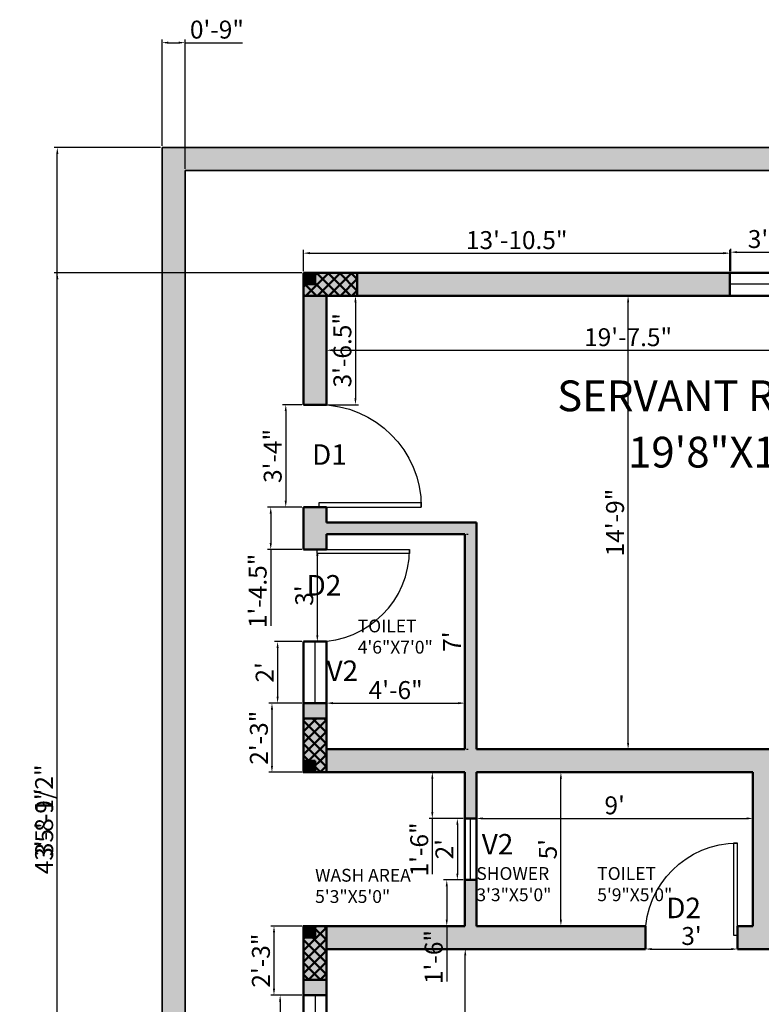
# Model space of a CAD drawing. Units: inches. Extents: x 1749 to 3550, y 1117 to 2383.
# Tile 7 of 15: x 1749 to 2038, y 1993 to 2377. Entities that reach past the tile are written whole.
import ezdxf

# ---------------------------------------------------------------- set-up
doc = ezdxf.new("R2010")
doc.units = ezdxf.units.IN
for name, color, linetype, lineweight in [('A-ANNO-DIMS', 2, 'Continuous', 18), ('A-ANNO-TEXT', 3, 'Continuous', 18), ('A-AREA-IDEN', 7, 'Continuous', 18), ('A-COLS', 10, 'Continuous', 50), ('A-DOOR', 30, 'Continuous', 25), ('A-GLAZ', 4, 'Continuous', 25), ('A-WALL', 7, 'Continuous', 50), ('A-WALL-PATT', 8, 'Continuous', 13), ('C-PROP', 8, 'Continuous', 35)]:
    doc.layers.add(name, color=color, linetype=linetype, lineweight=lineweight)
doc.styles.get("Standard").update_dxf_attribs({"font": 'arial.ttf'})
doc.dimstyles.new('ISO-25', dxfattribs={"dimtxt": 7, "dimasz": 2.5, "dimexe": 1.25, "dimexo": 0.625, "dimtad": 1, "dimdec": 1, "dimlunit": 3, "dimtxsty": 'Standard', "dimcen": 2.5, "dimadec": 0, "dimazin": 0, "dimtfac": 1, "dimtdec": 1, "dimtmove": 0, "dimatfit": 3, "dimfxl": 1, "dimarcsym": 0})

# ---------------------------------------------------------------- blocks, each defined once
blk = doc.blocks.new('*U2')
for p, q in [((0, 0), (0, -6)), ((40, 0), (40, -6))]:
    blk.add_line(p, q)
blk.add_lwpolyline([(0, 0), (0, 40), (1.75, 40), (1.75, 0)], close=True)
blk.add_arc((0, 0), 40, 0, 90)
blk = doc.blocks.new('*U3')
for p, q in [((0, 0), (0, -6)), ((40, 0), (40, -6))]:
    blk.add_line(p, q)
blk.add_lwpolyline([(0, 0), (0, 40), (1.75, 40), (1.75, 0)], close=True)
blk.add_arc((0, 0), 40, 0, 90)
blk = doc.blocks.new('*D4')
at = {"layer": 'A-ANNO-DIMS', "color": 0, "lineweight": -2, "transparency": 16777216}
for p, q in [((1994.36, 2269.66), (1985.1, 2269.66)), ((1986.35, 2095.16), (1986.35, 2267.16)), ((1994.36, 2092.66), (1985.1, 2092.66))]:
    blk.add_line(p, q, dxfattribs=at)
at = {"layer": 'A-ANNO-DIMS', "color": 0, "transparency": 16777216}
for points in [[(1985.94, 2267.16), (1986.77, 2267.16), (1986.35, 2269.66)], [(1985.94, 2095.16), (1986.77, 2095.16), (1986.35, 2092.66)]]:
    blk.add_solid(points, dxfattribs=at)
at = {"layer": 'Defpoints', "color": 0, "transparency": 16777216}
for p in [(1986.35, 2269.66), (1994.99, 2269.66), (1994.99, 2092.66)]:
    blk.add_point(p, dxfattribs=at)
at = {"layer": 'A-ANNO-DIMS', "color": 0, "transparency": 16777216, "insert": (1982.16, 2181.16), "char_height": 7, "attachment_point": 5, "rotation": 90}
blk.add_mtext('14\'-9"', dxfattribs=at)
blk = doc.blocks.new('*D5')
at = {"layer": 'A-ANNO-DIMS', "color": 0, "lineweight": -2, "transparency": 16777216}
for p, q in [((1868.6, 2249.04), (1868.6, 2249.66)), ((2104.1, 2249.04), (2104.1, 2249.66)), ((1871.1, 2248.41), (2101.6, 2248.41))]:
    blk.add_line(p, q, dxfattribs=at)
at = {"layer": 'A-ANNO-DIMS', "color": 0, "transparency": 16777216}
for points in [[(1871.1, 2248.83), (1871.1, 2247.99), (1868.6, 2248.41)], [(2101.6, 2248.83), (2101.6, 2247.99), (2104.1, 2248.41)]]:
    blk.add_solid(points, dxfattribs=at)
at = {"layer": 'Defpoints', "color": 0, "transparency": 16777216}
for p in [(1868.6, 2248.41), (2104.1, 2248.41), (2104.1, 2248.41)]:
    blk.add_point(p, dxfattribs=at)
at = {"layer": 'A-ANNO-DIMS', "color": 0, "transparency": 16777216, "insert": (1986.35, 2252.61), "char_height": 7, "attachment_point": 5}
blk.add_mtext('19\'-7.5"', dxfattribs=at)
blk = doc.blocks.new('*D6')
at = {"layer": 'A-ANNO-DIMS', "color": 0, "lineweight": -2, "transparency": 16777216}
for p, q in [((1923.39, 2014.66), (1924.02, 2014.66)), ((1922.77, 1861.16), (1922.77, 2012.16)), ((1923.39, 1858.66), (1924.02, 1858.66))]:
    blk.add_line(p, q, dxfattribs=at)
at = {"layer": 'A-ANNO-DIMS', "color": 0, "transparency": 16777216}
for points in [[(1922.35, 2012.16), (1923.18, 2012.16), (1922.77, 2014.66)], [(1922.35, 1861.16), (1923.18, 1861.16), (1922.77, 1858.66)]]:
    blk.add_solid(points, dxfattribs=at)
at = {"layer": 'Defpoints', "color": 0, "transparency": 16777216}
for p in [(1922.77, 2014.66), (1922.77, 2014.66), (1922.77, 1858.66)]:
    blk.add_point(p, dxfattribs=at)
at = {"layer": 'A-ANNO-DIMS', "color": 0, "transparency": 16777216, "insert": (1918.57, 1936.66), "char_height": 7, "attachment_point": 5, "rotation": 90}
blk.add_mtext("13'", dxfattribs=at)
blk = doc.blocks.new('*D8')
at = {"layer": 'A-ANNO-DIMS', "color": 0, "lineweight": -2, "transparency": 16777216}
for p, q in [((1960.73, 2083.66), (1961.35, 2083.66)), ((1960.1, 2026.16), (1960.1, 2081.16)), ((1960.73, 2023.66), (1961.35, 2023.66))]:
    blk.add_line(p, q, dxfattribs=at)
at = {"layer": 'A-ANNO-DIMS', "color": 0, "transparency": 16777216}
for points in [[(1959.69, 2081.16), (1960.52, 2081.16), (1960.1, 2083.66)], [(1959.69, 2026.16), (1960.52, 2026.16), (1960.1, 2023.66)]]:
    blk.add_solid(points, dxfattribs=at)
at = {"layer": 'Defpoints', "color": 0, "transparency": 16777216}
for p in [(1960.1, 2083.66), (1960.1, 2083.66), (1960.1, 2023.66)]:
    blk.add_point(p, dxfattribs=at)
at = {"layer": 'A-ANNO-DIMS', "color": 0, "transparency": 16777216, "insert": (1955.92, 2053.66), "char_height": 7, "attachment_point": 5, "rotation": 90}
blk.add_mtext("5'", dxfattribs=at)
blk = doc.blocks.new('*D9')
at = {"layer": 'A-ANNO-DIMS', "color": 0, "lineweight": -2, "transparency": 16777216}
for p, q in [((1927.1, 2066.29), (1927.1, 2066.91)), ((1929.6, 2065.66), (2032.6, 2065.66)), ((2035.1, 2066.29), (2035.1, 2066.91))]:
    blk.add_line(p, q, dxfattribs=at)
at = {"layer": 'A-ANNO-DIMS', "color": 0, "transparency": 16777216}
for points in [[(1929.6, 2066.08), (1929.6, 2065.24), (1927.1, 2065.66)], [(2032.6, 2066.08), (2032.6, 2065.24), (2035.1, 2065.66)]]:
    blk.add_solid(points, dxfattribs=at)
at = {"layer": 'Defpoints', "color": 0, "transparency": 16777216}
for p in [(1927.1, 2065.66), (2035.1, 2065.66), (2035.1, 2065.66)]:
    blk.add_point(p, dxfattribs=at)
at = {"layer": 'A-ANNO-DIMS', "color": 0, "transparency": 16777216, "insert": (1981.1, 2069.86), "char_height": 7, "attachment_point": 5}
blk.add_mtext("9'", dxfattribs=at)
blk = doc.blocks.new('*D10')
at = {"layer": 'A-ANNO-DIMS', "color": 0, "lineweight": -2, "transparency": 16777216}
for p, q in [((1923.23, 2176.66), (1923.85, 2176.66)), ((1922.6, 2095.16), (1922.6, 2174.16)), ((1923.23, 2092.66), (1923.85, 2092.66))]:
    blk.add_line(p, q, dxfattribs=at)
at = {"layer": 'A-ANNO-DIMS', "color": 0, "transparency": 16777216}
for points in [[(1922.19, 2174.16), (1923.02, 2174.16), (1922.6, 2176.66)], [(1922.19, 2095.16), (1923.02, 2095.16), (1922.6, 2092.66)]]:
    blk.add_solid(points, dxfattribs=at)
at = {"layer": 'Defpoints', "color": 0, "transparency": 16777216}
for p in [(1922.6, 2176.66), (1922.6, 2176.66), (1922.6, 2092.66)]:
    blk.add_point(p, dxfattribs=at)
at = {"layer": 'A-ANNO-DIMS', "color": 0, "transparency": 16777216, "insert": (1918.48, 2134.66), "char_height": 7, "attachment_point": 5, "rotation": 90}
blk.add_mtext("7'", dxfattribs=at)
blk = doc.blocks.new('*D11')
at = {"layer": 'A-ANNO-DIMS', "color": 0, "lineweight": -2, "transparency": 16777216}
for p, q in [((1868.6, 2111.29), (1868.6, 2111.91)), ((1871.1, 2110.66), (1920.1, 2110.66)), ((1922.6, 2111.29), (1922.6, 2111.91))]:
    blk.add_line(p, q, dxfattribs=at)
at = {"layer": 'A-ANNO-DIMS', "color": 0, "transparency": 16777216}
for points in [[(1871.1, 2111.08), (1871.1, 2110.24), (1868.6, 2110.66)], [(1920.1, 2111.08), (1920.1, 2110.24), (1922.6, 2110.66)]]:
    blk.add_solid(points, dxfattribs=at)
at = {"layer": 'Defpoints', "color": 0, "transparency": 16777216}
for p in [(1868.6, 2110.66), (1922.6, 2110.66), (1922.6, 2110.66)]:
    blk.add_point(p, dxfattribs=at)
at = {"layer": 'A-ANNO-DIMS', "color": 0, "transparency": 16777216, "insert": (1895.6, 2114.86), "char_height": 7, "attachment_point": 5}
blk.add_mtext('4\'-6"', dxfattribs=at)
blk = doc.blocks.new('*D75')
at = {"layer": 'A-ANNO-DIMS', "color": 0, "lineweight": -2, "ltscale": 0.5, "transparency": 16777216}
for p, q in [((1859.6, 2279.29), (1859.6, 2287.56)), ((2026.1, 2279.29), (2026.1, 2287.56)), ((1862.1, 2286.31), (2023.6, 2286.31))]:
    blk.add_line(p, q, dxfattribs=at)
at = {"layer": 'A-ANNO-DIMS', "color": 0, "ltscale": 0.5, "transparency": 16777216}
for points in [[(1862.1, 2286.73), (1862.1, 2285.9), (1859.6, 2286.31)], [(2023.6, 2286.73), (2023.6, 2285.9), (2026.1, 2286.31)]]:
    blk.add_solid(points, dxfattribs=at)
at = {"layer": 'Defpoints', "color": 0, "ltscale": 0.5, "transparency": 16777216}
for p in [(2026.1, 2286.31), (1859.6, 2278.66), (2026.1, 2278.66)]:
    blk.add_point(p, dxfattribs=at)
at = {"layer": 'A-ANNO-DIMS', "color": 0, "ltscale": 0.5, "transparency": 16777216, "insert": (1942.85, 2290.51), "char_height": 7, "attachment_point": 5}
blk.add_mtext('13\'-10.5"', dxfattribs=at)
blk = doc.blocks.new('*D76')
at = {"layer": 'A-ANNO-DIMS', "color": 0, "lineweight": -2, "ltscale": 0.5, "transparency": 16777216}
for p, q in [((2026.42, 2279.29), (2026.42, 2287.96)), ((2074.1, 2279.29), (2074.1, 2287.96)), ((2028.92, 2286.71), (2071.6, 2286.71))]:
    blk.add_line(p, q, dxfattribs=at)
at = {"layer": 'A-ANNO-DIMS', "color": 0, "ltscale": 0.5, "transparency": 16777216}
for points in [[(2028.92, 2287.12), (2028.92, 2286.29), (2026.42, 2286.71)], [(2071.6, 2287.12), (2071.6, 2286.29), (2074.1, 2286.71)]]:
    blk.add_solid(points, dxfattribs=at)
at = {"layer": 'Defpoints', "color": 0, "ltscale": 0.5, "transparency": 16777216}
for p in [(2074.1, 2286.71), (2026.42, 2278.66), (2074.1, 2278.66)]:
    blk.add_point(p, dxfattribs=at)
at = {"layer": 'A-ANNO-DIMS', "color": 0, "ltscale": 0.5, "transparency": 16777216, "insert": (2050.26, 2290.91), "char_height": 7, "attachment_point": 5}
blk.add_mtext('3\'-11.7"', dxfattribs=at)
blk = doc.blocks.new('*D78')
at = {"layer": 'A-ANNO-DIMS', "color": 0, "lineweight": -2, "ltscale": 0.5, "transparency": 16777216}
for p, q in [((1869.23, 2269.66), (1881.14, 2269.66)), ((1879.89, 2267.16), (1879.89, 2229.66)), ((1869.23, 2227.16), (1881.14, 2227.16))]:
    blk.add_line(p, q, dxfattribs=at)
at = {"layer": 'A-ANNO-DIMS', "color": 0, "ltscale": 0.5, "transparency": 16777216}
for points in [[(1879.48, 2267.16), (1880.31, 2267.16), (1879.89, 2269.66)], [(1879.48, 2229.66), (1880.31, 2229.66), (1879.89, 2227.16)]]:
    blk.add_solid(points, dxfattribs=at)
at = {"layer": 'Defpoints', "color": 0, "ltscale": 0.5, "transparency": 16777216}
for p in [(1868.6, 2269.66), (1868.6, 2227.16), (1879.89, 2227.16)]:
    blk.add_point(p, dxfattribs=at)
at = {"layer": 'A-ANNO-DIMS', "color": 0, "ltscale": 0.5, "transparency": 16777216, "insert": (1875.69, 2248.41), "char_height": 7, "attachment_point": 5, "rotation": 90}
blk.add_mtext('3\'-6.5"', dxfattribs=at)
blk = doc.blocks.new('*D79')
at = {"layer": 'A-ANNO-DIMS', "color": 0, "lineweight": -2, "ltscale": 0.5, "transparency": 16777216}
for p, q in [((1858.98, 2227.16), (1851.43, 2227.16)), ((1852.68, 2224.66), (1852.68, 2189.66)), ((1858.98, 2187.16), (1851.43, 2187.16))]:
    blk.add_line(p, q, dxfattribs=at)
at = {"layer": 'A-ANNO-DIMS', "color": 0, "ltscale": 0.5, "transparency": 16777216}
for points in [[(1852.26, 2224.66), (1853.09, 2224.66), (1852.68, 2227.16)], [(1852.26, 2189.66), (1853.09, 2189.66), (1852.68, 2187.16)]]:
    blk.add_solid(points, dxfattribs=at)
at = {"layer": 'Defpoints', "color": 0, "ltscale": 0.5, "transparency": 16777216}
for p in [(1859.61, 2227.16), (1852.68, 2187.16), (1859.6, 2187.16)]:
    blk.add_point(p, dxfattribs=at)
at = {"layer": 'A-ANNO-DIMS', "color": 0, "ltscale": 0.5, "transparency": 16777216, "insert": (1848.48, 2207.16), "char_height": 7, "attachment_point": 5, "rotation": 90}
blk.add_mtext('3\'-4"', dxfattribs=at)
blk = doc.blocks.new('*D80')
at = {"layer": 'A-ANNO-DIMS', "color": 0, "lineweight": -2, "ltscale": 0.5, "transparency": 16777216}
for p, q in [((1858.98, 2187.16), (1845.56, 2187.16)), ((1846.81, 2184.66), (1846.81, 2173.16)), ((1858.98, 2170.66), (1845.56, 2170.66)), ((1846.81, 2170.66), (1846.81, 2140.81))]:
    blk.add_line(p, q, dxfattribs=at)
at = {"layer": 'A-ANNO-DIMS', "color": 0, "ltscale": 0.5, "transparency": 16777216}
for points in [[(1846.39, 2184.66), (1847.23, 2184.66), (1846.81, 2187.16)], [(1846.39, 2173.16), (1847.23, 2173.16), (1846.81, 2170.66)]]:
    blk.add_solid(points, dxfattribs=at)
at = {"layer": 'Defpoints', "color": 0, "ltscale": 0.5, "transparency": 16777216}
for p in [(1859.6, 2187.16), (1846.81, 2170.66), (1859.6, 2170.66)]:
    blk.add_point(p, dxfattribs=at)
at = {"layer": 'A-ANNO-DIMS', "color": 0, "ltscale": 0.5, "transparency": 16777216, "insert": (1842.61, 2154.48), "char_height": 7, "attachment_point": 5, "rotation": 90}
blk.add_mtext('1\'-4.5"', dxfattribs=at)
blk = doc.blocks.new('*D81')
at = {"layer": 'A-ANNO-DIMS', "color": 0, "lineweight": -2, "ltscale": 0.5, "transparency": 16777216}
for p, q in [((1860.23, 2170.66), (1866.25, 2170.66)), ((1865, 2168.16), (1865, 2137.16)), ((1860.23, 2134.66), (1866.25, 2134.66))]:
    blk.add_line(p, q, dxfattribs=at)
at = {"layer": 'A-ANNO-DIMS', "color": 0, "ltscale": 0.5, "transparency": 16777216}
for points in [[(1864.59, 2168.16), (1865.42, 2168.16), (1865, 2170.66)], [(1864.59, 2137.16), (1865.42, 2137.16), (1865, 2134.66)]]:
    blk.add_solid(points, dxfattribs=at)
at = {"layer": 'Defpoints', "color": 0, "ltscale": 0.5, "transparency": 16777216}
for p in [(1859.6, 2170.66), (1859.6, 2134.66), (1865, 2134.66)]:
    blk.add_point(p, dxfattribs=at)
at = {"layer": 'A-ANNO-DIMS', "color": 0, "ltscale": 0.5, "transparency": 16777216, "insert": (1860.8, 2152.66), "char_height": 7, "attachment_point": 5, "rotation": 90}
blk.add_mtext("3'", dxfattribs=at)
blk = doc.blocks.new('*D82')
at = {"layer": 'A-ANNO-DIMS', "color": 0, "lineweight": -2, "ltscale": 0.5, "transparency": 16777216}
for p, q in [((1858.98, 2134.66), (1848.24, 2134.66)), ((1849.49, 2132.16), (1849.49, 2113.16)), ((1858.98, 2110.66), (1848.24, 2110.66))]:
    blk.add_line(p, q, dxfattribs=at)
at = {"layer": 'A-ANNO-DIMS', "color": 0, "ltscale": 0.5, "transparency": 16777216}
for points in [[(1849.08, 2132.16), (1849.91, 2132.16), (1849.49, 2134.66)], [(1849.08, 2113.16), (1849.91, 2113.16), (1849.49, 2110.66)]]:
    blk.add_solid(points, dxfattribs=at)
at = {"layer": 'Defpoints', "color": 0, "ltscale": 0.5, "transparency": 16777216}
for p in [(1859.6, 2134.66), (1849.49, 2110.66), (1859.6, 2110.66)]:
    blk.add_point(p, dxfattribs=at)
at = {"layer": 'A-ANNO-DIMS', "color": 0, "ltscale": 0.5, "transparency": 16777216, "insert": (1845.35, 2122.66), "char_height": 7, "attachment_point": 5, "rotation": 90}
blk.add_mtext("2'", dxfattribs=at)
blk = doc.blocks.new('*D83')
at = {"layer": 'A-ANNO-DIMS', "color": 0, "lineweight": -2, "ltscale": 0.5, "transparency": 16777216}
for p, q in [((1858.98, 2110.66), (1846.04, 2110.66)), ((1847.29, 2108.16), (1847.29, 2086.16)), ((1858.98, 2083.66), (1846.04, 2083.66))]:
    blk.add_line(p, q, dxfattribs=at)
at = {"layer": 'A-ANNO-DIMS', "color": 0, "ltscale": 0.5, "transparency": 16777216}
for points in [[(1846.87, 2108.16), (1847.71, 2108.16), (1847.29, 2110.66)], [(1846.87, 2086.16), (1847.71, 2086.16), (1847.29, 2083.66)]]:
    blk.add_solid(points, dxfattribs=at)
at = {"layer": 'Defpoints', "color": 0, "ltscale": 0.5, "transparency": 16777216}
for p in [(1859.6, 2110.66), (1847.29, 2083.66), (1859.6, 2083.66)]:
    blk.add_point(p, dxfattribs=at)
at = {"layer": 'A-ANNO-DIMS', "color": 0, "ltscale": 0.5, "transparency": 16777216, "insert": (1843.09, 2097.16), "char_height": 7, "attachment_point": 5, "rotation": 90}
blk.add_mtext('2\'-3"', dxfattribs=at)
blk = doc.blocks.new('*D84')
at = {"layer": 'A-ANNO-DIMS', "color": 0, "lineweight": -2, "ltscale": 0.5, "transparency": 16777216}
for p, q in [((1921.98, 2083.66), (1908.65, 2083.66)), ((1909.9, 2081.16), (1909.9, 2068.16)), ((1921.98, 2065.66), (1908.65, 2065.66)), ((1909.9, 2065.66), (1909.9, 2043.96))]:
    blk.add_line(p, q, dxfattribs=at)
at = {"layer": 'A-ANNO-DIMS', "color": 0, "ltscale": 0.5, "transparency": 16777216}
for points in [[(1909.49, 2081.16), (1910.32, 2081.16), (1909.9, 2083.66)], [(1909.49, 2068.16), (1910.32, 2068.16), (1909.9, 2065.66)]]:
    blk.add_solid(points, dxfattribs=at)
at = {"layer": 'Defpoints', "color": 0, "ltscale": 0.5, "transparency": 16777216}
for p in [(1922.6, 2083.66), (1909.9, 2065.66), (1922.6, 2065.66)]:
    blk.add_point(p, dxfattribs=at)
at = {"layer": 'A-ANNO-DIMS', "color": 0, "ltscale": 0.5, "transparency": 16777216, "insert": (1905.7, 2053.56), "char_height": 7, "attachment_point": 5, "rotation": 90}
blk.add_mtext('1\'-6"', dxfattribs=at)
blk = doc.blocks.new('*D85')
at = {"layer": 'A-ANNO-DIMS', "color": 0, "lineweight": -2, "ltscale": 0.5, "transparency": 16777216}
for p, q in [((1921.98, 2065.66), (1918.43, 2065.66)), ((1919.68, 2063.16), (1919.68, 2044.16)), ((1921.98, 2041.66), (1918.43, 2041.66))]:
    blk.add_line(p, q, dxfattribs=at)
at = {"layer": 'A-ANNO-DIMS', "color": 0, "ltscale": 0.5, "transparency": 16777216}
for points in [[(1919.26, 2063.16), (1920.1, 2063.16), (1919.68, 2065.66)], [(1919.26, 2044.16), (1920.1, 2044.16), (1919.68, 2041.66)]]:
    blk.add_solid(points, dxfattribs=at)
at = {"layer": 'Defpoints', "color": 0, "ltscale": 0.5, "transparency": 16777216}
for p in [(1922.6, 2065.66), (1919.68, 2041.66), (1922.6, 2041.66)]:
    blk.add_point(p, dxfattribs=at)
at = {"layer": 'A-ANNO-DIMS', "color": 0, "ltscale": 0.5, "transparency": 16777216, "insert": (1915.54, 2053.66), "char_height": 7, "attachment_point": 5, "rotation": 90}
blk.add_mtext("2'", dxfattribs=at)
blk = doc.blocks.new('*D86')
at = {"layer": 'A-ANNO-DIMS', "color": 0, "lineweight": -2, "ltscale": 0.5, "transparency": 16777216}
for p, q in [((1921.98, 2041.66), (1914.3, 2041.66)), ((1915.55, 2039.16), (1915.55, 2026.16)), ((1921.98, 2023.66), (1914.3, 2023.66)), ((1915.55, 2023.66), (1915.55, 2001.96))]:
    blk.add_line(p, q, dxfattribs=at)
at = {"layer": 'A-ANNO-DIMS', "color": 0, "ltscale": 0.5, "transparency": 16777216}
for points in [[(1915.14, 2039.16), (1915.97, 2039.16), (1915.55, 2041.66)], [(1915.14, 2026.16), (1915.97, 2026.16), (1915.55, 2023.66)]]:
    blk.add_solid(points, dxfattribs=at)
at = {"layer": 'Defpoints', "color": 0, "ltscale": 0.5, "transparency": 16777216}
for p in [(1922.6, 2041.66), (1915.55, 2023.66), (1922.6, 2023.66)]:
    blk.add_point(p, dxfattribs=at)
at = {"layer": 'A-ANNO-DIMS', "color": 0, "ltscale": 0.5, "transparency": 16777216, "insert": (1911.35, 2011.56), "char_height": 7, "attachment_point": 5, "rotation": 90}
blk.add_mtext('1\'-6"', dxfattribs=at)
blk = doc.blocks.new('*D87')
at = {"layer": 'A-ANNO-DIMS', "color": 0, "lineweight": -2, "ltscale": 0.5, "transparency": 16777216}
for p, q in [((1858.98, 2023.66), (1846.83, 2023.66)), ((1848.08, 2021.16), (1848.08, 1999.16)), ((1858.98, 1996.66), (1846.83, 1996.66))]:
    blk.add_line(p, q, dxfattribs=at)
at = {"layer": 'A-ANNO-DIMS', "color": 0, "ltscale": 0.5, "transparency": 16777216}
for points in [[(1847.66, 2021.16), (1848.5, 2021.16), (1848.08, 2023.66)], [(1847.66, 1999.16), (1848.5, 1999.16), (1848.08, 1996.66)]]:
    blk.add_solid(points, dxfattribs=at)
at = {"layer": 'Defpoints', "color": 0, "ltscale": 0.5, "transparency": 16777216}
for p in [(1859.6, 2023.66), (1848.08, 1996.66), (1859.6, 1996.66)]:
    blk.add_point(p, dxfattribs=at)
at = {"layer": 'A-ANNO-DIMS', "color": 0, "ltscale": 0.5, "transparency": 16777216, "insert": (1843.88, 2010.16), "char_height": 7, "attachment_point": 5, "rotation": 90}
blk.add_mtext('2\'-3"', dxfattribs=at)
blk = doc.blocks.new('*D88')
at = {"layer": 'A-ANNO-DIMS', "color": 0, "lineweight": -2, "ltscale": 0.5, "transparency": 16777216}
for p, q in [((1858.98, 1996.66), (1849.23, 1996.66)), ((1850.48, 1994.16), (1850.48, 1951.16)), ((1858.98, 1948.66), (1849.23, 1948.66))]:
    blk.add_line(p, q, dxfattribs=at)
at = {"layer": 'A-ANNO-DIMS', "color": 0, "ltscale": 0.5, "transparency": 16777216}
for points in [[(1850.06, 1994.16), (1850.89, 1994.16), (1850.48, 1996.66)], [(1850.06, 1951.16), (1850.89, 1951.16), (1850.48, 1948.66)]]:
    blk.add_solid(points, dxfattribs=at)
at = {"layer": 'Defpoints', "color": 0, "ltscale": 0.5, "transparency": 16777216}
for p in [(1859.6, 1996.66), (1850.48, 1948.66), (1859.6, 1948.66)]:
    blk.add_point(p, dxfattribs=at)
at = {"layer": 'A-ANNO-DIMS', "color": 0, "ltscale": 0.5, "transparency": 16777216, "insert": (1846.35, 1972.66), "char_height": 7, "attachment_point": 5, "rotation": 90}
blk.add_mtext("4'", dxfattribs=at)
blk = doc.blocks.new('*D99')
at = {"layer": 'A-ANNO-DIMS', "color": 0, "lineweight": -2, "ltscale": 0.5, "transparency": 16777216}
for p, q in [((1993.1, 2015.29), (1993.1, 2015.91)), ((1995.6, 2014.66), (2026.6, 2014.66)), ((2029.1, 2015.29), (2029.1, 2015.91))]:
    blk.add_line(p, q, dxfattribs=at)
at = {"layer": 'A-ANNO-DIMS', "color": 0, "ltscale": 0.5, "transparency": 16777216}
for points in [[(1995.6, 2015.08), (1995.6, 2014.24), (1993.1, 2014.66)], [(2026.6, 2015.08), (2026.6, 2014.24), (2029.1, 2014.66)]]:
    blk.add_solid(points, dxfattribs=at)
at = {"layer": 'Defpoints', "color": 0, "ltscale": 0.5, "transparency": 16777216}
for p in [(1993.1, 2014.66), (2029.1, 2014.66), (2029.1, 2014.66)]:
    blk.add_point(p, dxfattribs=at)
at = {"layer": 'A-ANNO-DIMS', "color": 0, "ltscale": 0.5, "transparency": 16777216, "insert": (2011.1, 2018.86), "char_height": 7, "attachment_point": 5}
blk.add_mtext("3'", dxfattribs=at)
blk = doc.blocks.new('*D158')
at = {"layer": 'A-ANNO-DIMS', "color": 0, "lineweight": -2, "ltscale": 0.5, "transparency": 16777216}
for p, q in [((1803.75, 2327.58), (1762.22, 2327.58)), ((1763.47, 1805.5), (1763.47, 2325.08)), ((1803.75, 1803), (1762.22, 1803))]:
    blk.add_line(p, q, dxfattribs=at)
at = {"layer": 'A-ANNO-DIMS', "color": 0, "ltscale": 0.5, "transparency": 16777216}
for points in [[(1763.05, 2325.08), (1763.89, 2325.08), (1763.47, 2327.58)], [(1763.05, 1805.5), (1763.89, 1805.5), (1763.47, 1803)]]:
    blk.add_solid(points, dxfattribs=at)
at = {"layer": 'Defpoints', "color": 0, "ltscale": 0.5, "transparency": 16777216}
for p in [(1763.47, 2327.58), (1804.37, 2327.58), (1804.37, 1803)]:
    blk.add_point(p, dxfattribs=at)
at = {"layer": 'A-ANNO-DIMS', "color": 0, "ltscale": 0.5, "transparency": 16777216, "insert": (1759.22, 2065.29), "char_height": 7, "attachment_point": 5, "rotation": 90}
blk.add_mtext('43\'-8 1/2"', dxfattribs=at)
blk = doc.blocks.new('*D159')
at = {"layer": 'A-ANNO-DIMS', "color": 0, "lineweight": -2, "ltscale": 0.5, "transparency": 16777216}
for p, q in [((1804.37, 2328.21), (1804.37, 2369.73)), ((1806.87, 2368.48), (1810.87, 2368.48)), ((1813.37, 2319.21), (1813.37, 2369.73)), ((1813.37, 2368.48), (1835.73, 2368.48))]:
    blk.add_line(p, q, dxfattribs=at)
at = {"layer": 'A-ANNO-DIMS', "color": 0, "ltscale": 0.5, "transparency": 16777216}
for points in [[(1806.87, 2368.9), (1806.87, 2368.06), (1804.37, 2368.48)], [(1810.87, 2368.9), (1810.87, 2368.06), (1813.37, 2368.48)]]:
    blk.add_solid(points, dxfattribs=at)
at = {"layer": 'Defpoints', "color": 0, "ltscale": 0.5, "transparency": 16777216}
for p in [(1813.37, 2368.48), (1804.37, 2327.58), (1813.37, 2318.58)]:
    blk.add_point(p, dxfattribs=at)
at = {"layer": 'A-ANNO-DIMS', "color": 0, "ltscale": 0.5, "transparency": 16777216, "insert": (1825.8, 2372.68), "char_height": 7, "attachment_point": 5}
blk.add_mtext('0\'-9"', dxfattribs=at)
blk = doc.blocks.new('*D163')
at = {"layer": 'A-ANNO-DIMS', "color": 0, "lineweight": -2, "ltscale": 0.5, "transparency": 16777216}
for p, q in [((1858.98, 2278.66), (1762.22, 2278.66)), ((1763.47, 1852.11), (1763.47, 2276.16)), ((1858.98, 1849.61), (1762.22, 1849.61))]:
    blk.add_line(p, q, dxfattribs=at)
at = {"layer": 'A-ANNO-DIMS', "color": 0, "ltscale": 0.5, "transparency": 16777216}
for points in [[(1763.05, 2276.16), (1763.89, 2276.16), (1763.47, 2278.66)], [(1763.05, 1852.11), (1763.89, 1852.11), (1763.47, 1849.61)]]:
    blk.add_solid(points, dxfattribs=at)
at = {"layer": 'Defpoints', "color": 0, "ltscale": 0.5, "transparency": 16777216}
for p in [(1763.47, 2278.66), (1859.6, 2278.66), (1859.6, 1849.61)]:
    blk.add_point(p, dxfattribs=at)
at = {"layer": 'A-ANNO-DIMS', "color": 0, "ltscale": 0.5, "transparency": 16777216, "insert": (1759.27, 2064.13), "char_height": 7, "attachment_point": 5, "rotation": 90}
blk.add_mtext('35\'-9"', dxfattribs=at)

msp = doc.modelspace()

# ---------------------------------------------------------------- hatches: boundary and pattern name
at = {"layer": 'A-COLS'}
h = msp.add_hatch(color=256, dxfattribs=at)
h.dxf.hatch_style = 1
h.paths.add_polyline_path([(1859.6, 2274.16), (1864.1, 2274.16), (1864.1, 2278.66), (1859.6, 2278.66)])
h = msp.add_hatch(dxfattribs=at)
h.set_pattern_fill('ANSI37', color=256)
h.set_pattern_definition([(45, (-386.9595, 498.1017), (-2.245064, 2.245064), []), (135, (-386.9595, 498.1017), (-2.245064, -2.245064), [])])
h.paths.add_polyline_path([(1880.6, 2278.66), (1859.6, 2278.66), (1859.6, 2269.66), (1880.6, 2269.66)])
h = msp.add_hatch(dxfattribs=at)
h.set_pattern_fill('ANSI37', color=256, angle=-90)
h.set_pattern_definition([(315, (88.0445, 4351.2253), (2.245064, 2.245064), []), (45, (88.0445, 4351.2253), (-2.245064, 2.245064), [])])
h.paths.add_polyline_path([(1868.6, 2104.66), (1859.6, 2104.66), (1859.6, 2083.66), (1868.6, 2083.66)])
h = msp.add_hatch(color=256, dxfattribs=at)
h.dxf.hatch_style = 1
h.paths.add_polyline_path([(1859.6, 2083.66), (1864.1, 2083.66), (1864.1, 2088.16), (1859.6, 2088.16)])
h = msp.add_hatch(color=256, dxfattribs=at)
h.dxf.hatch_style = 1
h.paths.add_polyline_path([(1859.6, 2019.16), (1864.1, 2019.16), (1864.1, 2023.66), (1859.6, 2023.66)])
h = msp.add_hatch(dxfattribs=at)
h.set_pattern_fill('ANSI37', color=256, angle=-90)
h.set_pattern_definition([(315, (88.0445, 4270.2253), (2.245064, 2.245064), []), (45, (88.0445, 4270.2253), (-2.245064, 2.245064), [])])
h.paths.add_polyline_path([(1868.6, 2023.66), (1859.6, 2023.66), (1859.6, 2002.66), (1868.6, 2002.66)])
at = {"layer": 'A-WALL-PATT', "ltscale": 0.5}
h = msp.add_hatch(color=256, dxfattribs=at)
h.dxf.hatch_style = 1
h.paths.add_polyline_path([(2612.84, 2327.58), (1804.37, 2327.58), (1804.37, 1803), (2612.84, 1803), (2612.84, 2093.66), (2603.84, 2093.66), (2603.84, 1812), (1813.37, 1812), (1813.37, 2318.58), (2603.84, 2318.58), (2603.84, 2268.45), (2612.84, 2268.45)])
at = {"layer": 'A-WALL-PATT'}
h = msp.add_hatch(color=256, dxfattribs=at)
h.dxf.hatch_style = 1
h.paths.add_polyline_path([(2026.1, 2278.66), (1859.6, 2278.66), (1859.6, 2227.16), (1868.6, 2227.16), (1868.6, 2269.66), (2026.1, 2269.66)])
h = msp.add_hatch(color=256, dxfattribs=at)
h.dxf.hatch_style = 1
h.paths.add_polyline_path([(2113.1, 2092.66), (2104.1, 2092.66), (1927.1, 2092.66), (1927.1, 2181.16), (1868.6, 2181.16), (1868.6, 2187.16), (1859.6, 2187.16), (1859.6, 2170.66), (1868.6, 2170.66), (1868.6, 2176.66), (1922.6, 2176.66), (1922.6, 2092.66), (1868.6, 2092.66), (1868.6, 2110.66), (1859.6, 2110.66), (1859.6, 2083.66), (1922.6, 2083.66), (1922.6, 2065.66), (1927.1, 2065.66), (1927.1, 2083.66), (2035.1, 2083.66), (2035.1, 2023.66), (2029.1, 2023.66), (2029.1, 2014.66), (2053.1, 2014.66), (2053.1, 2023.66), (2044.1, 2023.66), (2044.1, 2083.66), (2104.1, 2083.66), (2104.1, 2023.66), (2095.1, 2023.66), (2095.1, 2014.66), (2104.1, 2014.66), (2104.1, 1996.66), (2113.1, 1996.66)])
h = msp.add_hatch(color=256, dxfattribs=at)
h.dxf.hatch_style = 1
h.paths.add_polyline_path([(1993.1, 2023.66), (1927.1, 2023.66), (1927.1, 2041.66), (1922.6, 2041.66), (1922.6, 2023.66), (1859.6, 2023.66), (1859.6, 1996.66), (1868.6, 1996.66), (1868.6, 2014.66), (1993.1, 2014.66)])

# ---------------------------------------------------------------- linework, layer by layer
at = {"layer": 'A-COLS'}
for p, q in [((1859.6, 2278.66), (1859.6, 2274.16)), ((1864.1, 2278.66), (1859.6, 2278.66)), ((1864.1, 2274.16), (1864.1, 2278.66)), ((1859.6, 2274.16), (1864.1, 2274.16)), ((1859.6, 2088.16), (1859.6, 2083.66)), ((1864.1, 2088.16), (1859.6, 2088.16)), ((1864.1, 2083.66), (1864.1, 2088.16)), ((1859.6, 2083.66), (1864.1, 2083.66)), ((1859.6, 2023.66), (1859.6, 2019.16)), ((1864.1, 2023.66), (1859.6, 2023.66)), ((1864.1, 2019.16), (1864.1, 2023.66)), ((1859.6, 2019.16), (1864.1, 2019.16))]:
    msp.add_line(p, q, dxfattribs=at)
for points in [[(1859.6, 2278.66), (1880.6, 2278.66), (1880.6, 2269.66), (1859.6, 2269.66)], [(1868.6, 2104.66), (1868.6, 2083.66), (1859.6, 2083.66), (1859.6, 2104.66)], [(1868.6, 2023.66), (1868.6, 2002.66), (1859.6, 2002.66), (1859.6, 2023.66)]]:
    msp.add_lwpolyline(points, close=True, dxfattribs=at)
at = {"layer": 'A-GLAZ'}
for p, q in [((2074.1, 2274.16), (2026.1, 2274.16)), ((1864.1, 1996.66), (1864.1, 1948.66))]:
    msp.add_line(p, q, dxfattribs=at)
at = {"layer": 'A-GLAZ', "ltscale": 0.3}
for p, q in [((1864.1, 2110.66), (1864.1, 2134.66)), ((1924.85, 2041.66), (1924.85, 2065.66))]:
    msp.add_line(p, q, dxfattribs=at)
at = {"layer": 'A-WALL'}
for p, q in [((1859.6, 2278.66), (2113.1, 2278.66)), ((1859.6, 2278.66), (1859.6, 2227.16)), ((2026.1, 2269.66), (2026.1, 2278.66)), ((1868.6, 2269.66), (2104.1, 2269.66)), ((1868.6, 2269.66), (1868.6, 2227.16)), ((1868.6, 2227.16), (1859.6, 2227.16)), ((1859.6, 2187.16), (1859.6, 2170.66)), ((1868.6, 2187.16), (1859.6, 2187.16)), ((1868.6, 2187.16), (1868.6, 2181.16)), ((1868.6, 2181.16), (1927.1, 2181.16)), ((1927.1, 2181.16), (1927.1, 2092.66)), ((1868.6, 2176.66), (1922.6, 2176.66)), ((1868.6, 2176.66), (1868.6, 2170.66)), ((1922.6, 2176.66), (1922.6, 2092.66)), ((1868.6, 2170.66), (1859.6, 2170.66)), ((1859.6, 2134.66), (1859.6, 2083.66)), ((1868.6, 2134.66), (1859.6, 2134.66)), ((1868.6, 2134.66), (1868.6, 2092.66)), ((1868.6, 2110.66), (1859.6, 2110.66)), ((1868.6, 2092.66), (1922.6, 2092.66)), ((1927.1, 2092.66), (2104.1, 2092.66)), ((1859.6, 2083.66), (1922.6, 2083.66)), ((1922.6, 2083.66), (1922.6, 2023.66)), ((1927.1, 2083.66), (2035.1, 2083.66)), ((1927.1, 2083.66), (1927.1, 2023.66)), ((2035.1, 2083.66), (2035.1, 2023.66)), ((1922.6, 2065.66), (1927.1, 2065.66)), ((1922.6, 2041.66), (1927.1, 2041.66)), ((1859.6, 2023.66), (1922.6, 2023.66)), ((1859.6, 2023.66), (1859.6, 1849.66)), ((1927.1, 2023.66), (1993.1, 2023.66)), ((1993.1, 2023.66), (1993.1, 2014.66)), ((2029.1, 2023.66), (2035.1, 2023.66)), ((2029.1, 2023.66), (2029.1, 2014.66)), ((1868.6, 2014.66), (1993.1, 2014.66)), ((1868.6, 2014.66), (1868.6, 1858.66)), ((2029.1, 2014.66), (2053.1, 2014.66)), ((1868.6, 1996.66), (1859.6, 1996.66))]:
    msp.add_line(p, q, dxfattribs=at)
at = {"layer": 'C-PROP', "ltscale": 0.5}
for p, q in [((1804.37, 1803), (1804.37, 2327.58)), ((1804.37, 2327.58), (2612.84, 2327.58)), ((1813.37, 1812), (1813.37, 2318.58)), ((1813.37, 2318.58), (2603.84, 2318.58))]:
    msp.add_line(p, q, dxfattribs=at)

# ---------------------------------------------------------------- block references
at = {"layer": 'A-DOOR', "xscale": -1, "rotation": 270}
msp.add_blockref('*U3', (1865.61, 2187.16), dxfattribs=at)
at = {"layer": 'A-DOOR', "xscale": 0.9, "yscale": 0.9, "zscale": 0.9, "rotation": 270}
msp.add_blockref('*U2', (1865, 2170.66), dxfattribs=at)
at = {"layer": 'A-DOOR', "xscale": -0.9, "yscale": 0.9, "zscale": 0.9}
msp.add_blockref('*U2', (2029.1, 2020.06), dxfattribs=at)

# ---------------------------------------------------------------- texts
at = {"layer": 'A-ANNO-TEXT', "ltscale": 0.5}
for s, p in [('D1', (1862.93, 2203.69)), ('D2', (1860.8, 2152.66)), ('V2', (1868.6, 2119.29)), ('V2', (1929.21, 2051.58)), ('D2', (2001.23, 2026.72))]:
    msp.add_text(s, height=8, dxfattribs=at).set_placement(p)
at = {"layer": 'A-AREA-IDEN', "ltscale": 0.5}
msp.add_text('SERVANT ROOM', height=12, rotation=0.0333, dxfattribs=at).set_placement((1958.68, 2224.61))
for s, height, p in [('19\'8"X14\'9"', 12, (1986.35, 2202.64)), ('TOILET', 5, (1880.78, 2138.3)), ('4\'6"X7\'0"', 5, (1880.78, 2130)), ('WASH AREA', 5, (1864.15, 2040.97)), ('SHOWER', 5, (1927.1, 2041.66)), ('TOILET', 5, (1974.3, 2041.66)), ('5\'3"X5\'0"', 5, (1864.15, 2032.67)), ('3\'3"X5\'0"', 5, (1927.1, 2033.36)), ('5\'9"X5\'0"', 5, (1974.3, 2033.36))]:
    msp.add_text(s, height=height, dxfattribs=at).set_placement(p)

# ---------------------------------------------------------------- dimensions: what is measured, and where the dimension line sits
at = {"layer": 'A-ANNO-DIMS', "ltscale": 0.5}
for base, p1, p2, override, picture, middle in [((1813.37, 2368.48), (1804.37, 2327.58), (1813.37, 2318.58), {"dimdec": 1, "dimlfac": 1, "dimrnd": 0, "dimzin": 1, "dimdsep": 46, "dimlunit": 4, "dimfrac": 2}, '*D159', (1825.8, 2372.68)), ((2026.1, 2286.31), (1859.6, 2278.66), (2026.1, 2278.66), {"dimclrd": 0, "dimclre": 0, "dimclrt": 0}, '*D75', (1942.85, 2290.51)), ((2074.1, 2286.71), (2026.42, 2278.66), (2074.1, 2278.66), {"dimclrd": 0, "dimclre": 0, "dimclrt": 0}, '*D76', (2050.26, 2290.91)), ((2029.1, 2014.66), (1993.1, 2014.66), (2029.1, 2014.66), {"dimclrd": 0, "dimclre": 0, "dimclrt": 0}, '*D99', (2011.1, 2018.86))]:
    dim = msp.add_linear_dim(base=base, p1=p1, p2=p2, dimstyle='ISO-25', override=override, dxfattribs=at)
    dim.commit()
    dim.dimension.update_dxf_attribs({"geometry": picture, "text_midpoint": middle})
for base, p1, p2, override, picture, middle in [((1763.47, 2327.58), (1804.37, 1803), (1804.37, 2327.58), {"dimdec": 1, "dimlfac": 1, "dimrnd": 0, "dimzin": 1, "dimdsep": 46, "dimlunit": 4, "dimfrac": 2}, '*D158', (1759.22, 2065.29)), ((1763.4701, 2278.6615), (1859.6043, 1849.6077), (1859.6043, 2278.6615), {"dimdec": 1, "dimlfac": 1, "dimrnd": 0, "dimzin": 1, "dimdsep": 46, "dimlunit": 4, "dimfrac": 2}, '*D163', (1759.2687, 2064.1346)), ((1879.89, 2227.16), (1868.6, 2269.66), (1868.6, 2227.16), {"dimclrd": 0, "dimclre": 0, "dimclrt": 0}, '*D78', (1875.69, 2248.41)), ((1852.68, 2187.16), (1859.61, 2227.16), (1859.6, 2187.16), {"dimclrd": 0, "dimclre": 0, "dimclrt": 0}, '*D79', (1848.48, 2207.16)), ((1846.81, 2170.66), (1859.6, 2187.16), (1859.6, 2170.66), {"dimclrd": 0, "dimclre": 0, "dimclrt": 0}, '*D80', (1842.61, 2154.48)), ((1865, 2134.66), (1859.6, 2170.66), (1859.6, 2134.66), {"dimclrd": 0, "dimclre": 0, "dimclrt": 0}, '*D81', (1860.8, 2152.66)), ((1849.49, 2110.66), (1859.6, 2134.66), (1859.6, 2110.66), {"dimclrd": 0, "dimclre": 0, "dimclrt": 0}, '*D82', (1845.35, 2122.66)), ((1847.29, 2083.66), (1859.6, 2110.66), (1859.6, 2083.66), {"dimclrd": 0, "dimclre": 0, "dimclrt": 0}, '*D83', (1843.09, 2097.16)), ((1909.9, 2065.66), (1922.6, 2083.66), (1922.6, 2065.66), {"dimclrd": 0, "dimclre": 0, "dimclrt": 0}, '*D84', (1905.7, 2053.56)), ((1919.68, 2041.66), (1922.6, 2065.66), (1922.6, 2041.66), {"dimclrd": 0, "dimclre": 0, "dimclrt": 0}, '*D85', (1915.54, 2053.66)), ((1915.55, 2023.66), (1922.6, 2041.66), (1922.6, 2023.66), {"dimclrd": 0, "dimclre": 0, "dimclrt": 0}, '*D86', (1911.35, 2011.56)), ((1848.08, 1996.66), (1859.6, 2023.66), (1859.6, 1996.66), {"dimclrd": 0, "dimclre": 0, "dimclrt": 0}, '*D87', (1843.88, 2010.16)), ((1850.48, 1948.66), (1859.6, 1996.66), (1859.6, 1948.66), {"dimclrd": 0, "dimclre": 0, "dimclrt": 0}, '*D88', (1846.35, 1972.66))]:
    dim = msp.add_linear_dim(base=base, p1=p1, p2=p2, angle=90, dimstyle='ISO-25', override=override, dxfattribs=at)
    dim.commit()
    dim.dimension.update_dxf_attribs({"geometry": picture, "text_midpoint": middle})
at = {"layer": 'A-ANNO-DIMS'}
for base, p1, p2, picture, middle in [((1986.35, 2269.66), (1994.99, 2092.66), (1994.99, 2269.66), '*D4', (1982.16, 2181.16)), ((1922.6, 2176.66), (1922.6, 2092.66), (1922.6, 2176.66), '*D10', (1918.48, 2134.66)), ((1960.1, 2083.66), (1960.1, 2023.66), (1960.1, 2083.66), '*D8', (1955.92, 2053.66)), ((1922.77, 2014.66), (1922.77, 1858.66), (1922.77, 2014.66), '*D6', (1918.57, 1936.66))]:
    dim = msp.add_linear_dim(base=base, p1=p1, p2=p2, angle=90, dimstyle='ISO-25', override={"dimclrd": 0, "dimclre": 0, "dimclrt": 0}, dxfattribs=at)
    dim.commit()
    dim.dimension.update_dxf_attribs({"geometry": picture, "text_midpoint": middle})
for base, p1, p2, picture, middle in [((2104.1, 2248.41), (1868.6, 2248.41), (2104.1, 2248.41), '*D5', (1986.35, 2252.61)), ((1922.6, 2110.66), (1868.6, 2110.66), (1922.6, 2110.66), '*D11', (1895.6, 2114.86)), ((2035.1, 2065.66), (1927.1, 2065.66), (2035.1, 2065.66), '*D9', (1981.1, 2069.86))]:
    dim = msp.add_linear_dim(base=base, p1=p1, p2=p2, dimstyle='ISO-25', override={"dimclrd": 0, "dimclre": 0, "dimclrt": 0}, dxfattribs=at)
    dim.commit()
    dim.dimension.update_dxf_attribs({"geometry": picture, "text_midpoint": middle})

doc.saveas('drawing.dxf')
